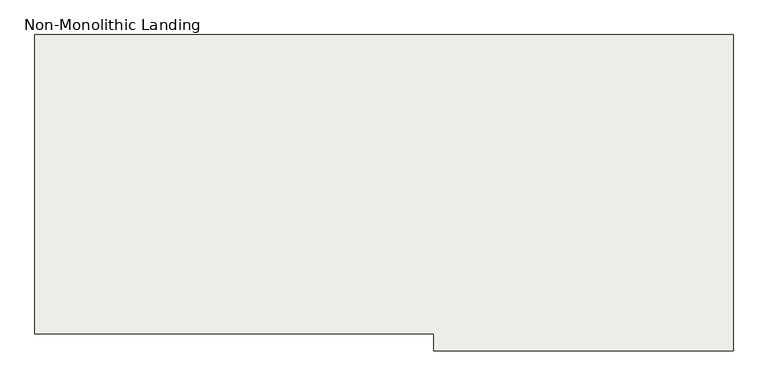
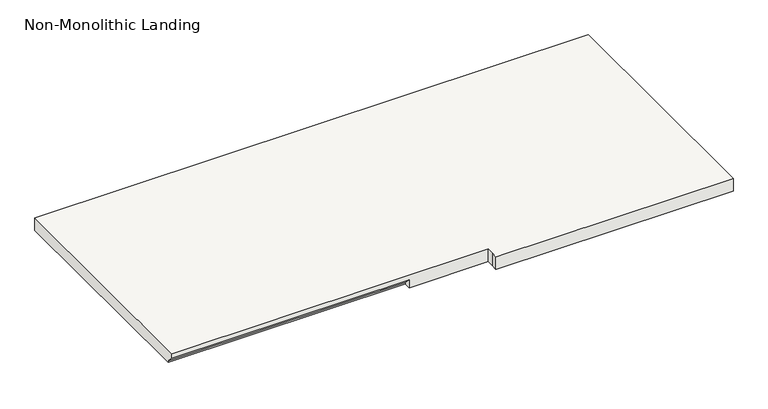
"""IFC4 building model written with IfcOpenShell, lengths in millimetres: slab geometry, Non-Monolithic Landing."""

from ifc_helpers import new_model, si_unit, origin, place, context, project, spatial, faceted_brep, source, transform, mapped, element, save


def non_monolithic_landing_cef278ae(model_context):
    return source(origin(), model_context, "Body", "Brep", [
        faceted_brep([(7464.4260838, 825.5660813, 5568.95), (7464.4260838, 850.9660813, 5543.55), (8378.8260838, 850.9660813, 5543.55), (8378.8260838, 825.5660813, 5568.95), (8683.6260838, 825.5660813, 5588.0), (8683.6260838, 798.8027016, 5588.0), (8683.6260838, 773.4027016, 5588.0), (9598.0260838, 773.4027016, 5588.0), (9598.0260838, 798.8027016, 5588.0), (9598.0260838, 1739.9660813, 5588.0), (7464.4260838, 1739.9660813, 5588.0), (7464.4260838, 825.5660813, 5588.0), (8378.8260838, 850.9660813, 5537.2), (7464.4260838, 850.9660813, 5537.2), (7464.4260838, 1739.9660813, 5537.2), (9598.0260838, 1739.9660813, 5537.2), (9598.0260838, 798.8027016, 5537.2), (9598.0260838, 773.4027016, 5537.2), (8683.6260838, 773.4027016, 5537.2), (8683.6260838, 798.8027016, 5537.2), (8683.6260838, 825.5660813, 5537.2), (8378.8260838, 825.5660813, 5537.2)], [[[0, 1, 2, 3]], [[4, 5, 6, 7, 8, 9, 10, 11]], [[12, 13, 14, 15, 16, 17, 18, 19, 20, 21]], [[13, 12, 2, 1]], [[12, 21, 3, 2]], [[4, 11, 0, 3, 21, 20]], [[5, 4, 20, 19]], [[6, 5, 19, 18]], [[7, 6, 18, 17]], [[8, 7, 17, 16]], [[9, 8, 16, 15]], [[10, 9, 15, 14]], [[11, 10, 14, 13, 1, 0]]]),
    ])


if __name__ == "__main__":
    model = new_model("IFC4")
    model_context = context("Model", 3, world=origin())
    ifc_project = project(units=[si_unit("LENGTHUNIT", "METRE", prefix="MILLI")], contexts=[model_context])
    site = spatial("IfcSite", under=ifc_project)
    building = spatial("IfcBuilding", under=site)
    placement = place(None, origin())
    non_monolithic_landing_shape = non_monolithic_landing_cef278ae(model_context)
    element("IfcSlab", 1, ObjectType="Non-Monolithic Landing", at=placement, inside=building, context=model_context, shape_type="MappedRepresentation", body=[
        mapped(non_monolithic_landing_shape, transform((0.0, 0.0, 0.0), x_axis=(1.0, 0.0, 0.0), y_axis=(0.0, 1.0, 0.0), z_axis=(0.0, 0.0, 1.0))),
    ])
    save(model, "model.ifc")
